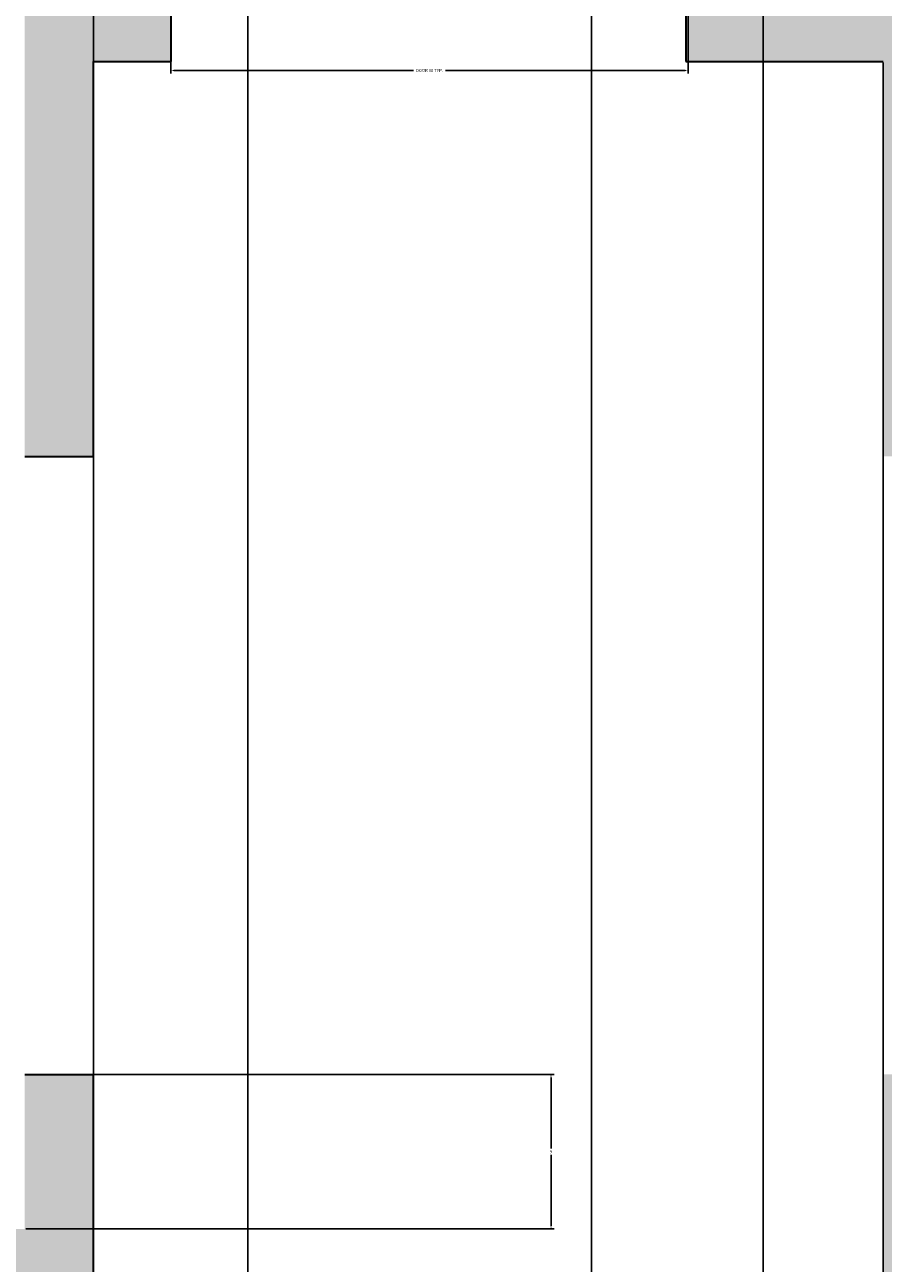
# Model space of a CAD drawing. Units: inches. Extents: x 1567 to 1964, y 1813 to 2447.
# Tile 24 of 28: x 1738 to 1788, y 2261 to 2333. Entities that reach past the tile are written whole.
import ezdxf

# ---------------------------------------------------------------- set-up
doc = ezdxf.new("R2010")
doc.units = ezdxf.units.IN
doc.layers.add('A-ANNO-DIMS', color=2, linetype='Continuous', lineweight=18)
doc.layers.add('A-WALL', color=7, linetype='Continuous', lineweight=35)
doc.layers.add('A-WALL-PATT', color=251, linetype='Continuous', lineweight=13, true_color=0x636466)
doc.styles.get("Standard").update_dxf_attribs({"font": 'arial.ttf'})
doc.dimstyles.get("Standard").update_dxf_attribs({"dimtxt": 0.18, "dimasz": 0.18, "dimexe": 0.18, "dimexo": 0.0625, "dimgap": 0.09, "dimtad": 0, "dimtih": 1, "dimtoh": 1, "dimdec": 4, "dimzin": 0, "dimdsep": 46, "dimtxsty": 'Standard', "dimcen": 0.09, "dimadec": 0, "dimazin": 0, "dimtfac": 1, "dimtdec": 4, "dimtofl": 0, "dimtmove": 0, "dimatfit": 3, "dimfxl": 1, "dimtolj": 1, "dimtzin": 0, "dimarcsym": 0})

# ---------------------------------------------------------------- blocks, each defined once
blk = doc.blocks.new('*D31')
at = {"layer": 'A-ANNO-DIMS', "color": 0, "lineweight": -2, "transparency": 16777216}
for p, q in [((1746.93, 2335.227), (1746.93, 2330.59)), ((1777.065, 2335.227), (1777.065, 2330.59)), ((1747.11, 2330.77), (1761.062, 2330.77)), ((1776.885, 2330.77), (1762.933, 2330.77))]:
    blk.add_line(p, q, dxfattribs=at)
at = {"layer": 'A-ANNO-DIMS', "color": 0, "transparency": 16777216}
for points in [[(1747.11, 2330.8), (1747.11, 2330.74), (1746.93, 2330.77)], [(1776.885, 2330.8), (1776.885, 2330.74), (1777.065, 2330.77)]]:
    blk.add_solid(points, dxfattribs=at)
at = {"layer": 'Defpoints', "color": 0, "transparency": 16777216}
for p in [(1746.93, 2335.29), (1777.065, 2335.29), (1777.065, 2330.77)]:
    blk.add_point(p, dxfattribs=at)
at = {"layer": 'A-ANNO-DIMS', "color": 0, "transparency": 16777216, "insert": (1761.997, 2330.77), "char_height": 0.18, "attachment_point": 5}
blk.add_mtext('\\A1;DOOR 30 TYP.', dxfattribs=at)
blk = doc.blocks.new('*D47')
at = {"layer": 'A-ANNO-DIMS', "color": 0, "lineweight": -2, "transparency": 16777216}
for p, q in [((1742.43, 2331.227), (1742.43, 1813.46)), ((1788.43, 2331.227), (1788.43, 1813.46)), ((1742.61, 1813.64), (1765.207, 1813.64)), ((1788.25, 1813.64), (1765.652, 1813.64))]:
    blk.add_line(p, q, dxfattribs=at)
at = {"layer": 'A-ANNO-DIMS', "color": 0, "transparency": 16777216}
for points in [[(1742.61, 1813.67), (1742.61, 1813.61), (1742.43, 1813.64)], [(1788.25, 1813.67), (1788.25, 1813.61), (1788.43, 1813.64)]]:
    blk.add_solid(points, dxfattribs=at)
at = {"layer": 'Defpoints', "color": 0, "transparency": 16777216}
for p in [(1742.43, 2331.29), (1788.43, 2331.29), (1788.43, 1813.64)]:
    blk.add_point(p, dxfattribs=at)
at = {"layer": 'A-ANNO-DIMS', "color": 0, "transparency": 16777216, "insert": (1765.43, 1813.64), "char_height": 0.18, "attachment_point": 5}
blk.add_mtext('\\A1;46', dxfattribs=at)
blk = doc.blocks.new('*D54')
at = {"layer": 'A-ANNO-DIMS', "color": 0, "lineweight": -2, "transparency": 16777216}
for p, q in [((1711.43, 1964.352), (1711.43, 2447.12)), ((1795.43, 1964.352), (1795.43, 2447.12)), ((1711.61, 2446.94), (1753.211, 2446.94)), ((1795.25, 2446.94), (1753.648, 2446.94))]:
    blk.add_line(p, q, dxfattribs=at)
at = {"layer": 'A-ANNO-DIMS', "color": 0, "transparency": 16777216}
for points in [[(1711.61, 2446.97), (1711.61, 2446.91), (1711.43, 2446.94)], [(1795.25, 2446.97), (1795.25, 2446.91), (1795.43, 2446.94)]]:
    blk.add_solid(points, dxfattribs=at)
at = {"layer": 'Defpoints', "color": 0, "transparency": 16777216}
for p in [(1795.43, 2446.94), (1711.43, 1964.29), (1795.43, 1964.29)]:
    blk.add_point(p, dxfattribs=at)
at = {"layer": 'A-ANNO-DIMS', "color": 0, "transparency": 16777216, "insert": (1753.43, 2446.94), "char_height": 0.18, "attachment_point": 5}
blk.add_mtext('\\A1;84', dxfattribs=at)
blk = doc.blocks.new('*D58')
at = {"layer": 'A-ANNO-DIMS', "color": 0, "lineweight": -2, "transparency": 16777216}
for p, q in [((1742.43, 2127.352), (1742.43, 2447.12)), ((1751.43, 2127.352), (1751.43, 2447.12)), ((1742.61, 2446.94), (1746.78, 2446.94)), ((1751.25, 2446.94), (1747.079, 2446.94))]:
    blk.add_line(p, q, dxfattribs=at)
at = {"layer": 'A-ANNO-DIMS', "color": 0, "transparency": 16777216}
for points in [[(1742.61, 2446.97), (1742.61, 2446.91), (1742.43, 2446.94)], [(1751.25, 2446.97), (1751.25, 2446.91), (1751.43, 2446.94)]]:
    blk.add_solid(points, dxfattribs=at)
at = {"layer": 'Defpoints', "color": 0, "transparency": 16777216}
for p in [(1751.43, 2446.94), (1742.43, 2127.29), (1751.43, 2127.29)]:
    blk.add_point(p, dxfattribs=at)
at = {"layer": 'A-ANNO-DIMS', "color": 0, "transparency": 16777216, "insert": (1746.93, 2446.94), "char_height": 0.18, "attachment_point": 5}
blk.add_mtext('\\A1;9', dxfattribs=at)
blk = doc.blocks.new('*D59')
at = {"layer": 'A-ANNO-DIMS', "color": 0, "lineweight": -2, "transparency": 16777216}
for p, q in [((1751.43, 2127.352), (1751.43, 2447.12)), ((1781.43, 2127.352), (1781.43, 2447.12)), ((1751.61, 2446.94), (1766.211, 2446.94)), ((1781.25, 2446.94), (1766.648, 2446.94))]:
    blk.add_line(p, q, dxfattribs=at)
at = {"layer": 'A-ANNO-DIMS', "color": 0, "transparency": 16777216}
for points in [[(1751.61, 2446.97), (1751.61, 2446.91), (1751.43, 2446.94)], [(1781.25, 2446.97), (1781.25, 2446.91), (1781.43, 2446.94)]]:
    blk.add_solid(points, dxfattribs=at)
at = {"layer": 'Defpoints', "color": 0, "transparency": 16777216}
for p in [(1781.43, 2446.94), (1751.43, 2127.29), (1781.43, 2127.29)]:
    blk.add_point(p, dxfattribs=at)
at = {"layer": 'A-ANNO-DIMS', "color": 0, "transparency": 16777216, "insert": (1766.43, 2446.94), "char_height": 0.18, "attachment_point": 5}
blk.add_mtext('\\A1;30', dxfattribs=at)
blk = doc.blocks.new('*D63')
at = {"layer": 'A-ANNO-DIMS', "color": 0, "lineweight": -2, "transparency": 16777216}
for p, q in [((1735.43, 1988.352), (1735.43, 2447.12)), ((1771.43, 1988.352), (1771.43, 2447.12)), ((1735.61, 2446.94), (1753.211, 2446.94)), ((1771.25, 2446.94), (1753.648, 2446.94))]:
    blk.add_line(p, q, dxfattribs=at)
at = {"layer": 'A-ANNO-DIMS', "color": 0, "transparency": 16777216}
for points in [[(1735.61, 2446.97), (1735.61, 2446.91), (1735.43, 2446.94)], [(1771.25, 2446.97), (1771.25, 2446.91), (1771.43, 2446.94)]]:
    blk.add_solid(points, dxfattribs=at)
at = {"layer": 'Defpoints', "color": 0, "transparency": 16777216}
for p in [(1771.43, 2446.94), (1735.43, 1988.29), (1771.43, 1988.29)]:
    blk.add_point(p, dxfattribs=at)
at = {"layer": 'A-ANNO-DIMS', "color": 0, "transparency": 16777216, "insert": (1753.43, 2446.94), "char_height": 0.18, "attachment_point": 5}
blk.add_mtext('\\A1;36', dxfattribs=at)
blk = doc.blocks.new('*D68')
at = {"layer": 'A-ANNO-DIMS', "color": 0, "lineweight": -2, "transparency": 16777216}
for p, q in [((1738.492, 2272.29), (1769.26, 2272.29)), ((1769.08, 2272.11), (1769.08, 2267.972)), ((1769.08, 2263.47), (1769.08, 2267.608)), ((1738.492, 2263.29), (1769.26, 2263.29))]:
    blk.add_line(p, q, dxfattribs=at)
at = {"layer": 'A-ANNO-DIMS', "color": 0, "transparency": 16777216}
for points in [[(1769.05, 2272.11), (1769.11, 2272.11), (1769.08, 2272.29)], [(1769.05, 2263.47), (1769.11, 2263.47), (1769.08, 2263.29)]]:
    blk.add_solid(points, dxfattribs=at)
at = {"layer": 'Defpoints', "color": 0, "transparency": 16777216}
for p in [(1738.43, 2272.29), (1738.43, 2263.29), (1769.08, 2263.29)]:
    blk.add_point(p, dxfattribs=at)
at = {"layer": 'A-ANNO-DIMS', "color": 0, "transparency": 16777216, "insert": (1769.08, 2267.79), "char_height": 0.18, "attachment_point": 5}
blk.add_mtext('\\A1;9', dxfattribs=at)

msp = doc.modelspace()

# ---------------------------------------------------------------- hatches: boundary and pattern name
at = {"layer": 'A-WALL-PATT'}
h = msp.add_hatch(color=256, dxfattribs=at)
h.dxf.hatch_style = 1
h.paths.add_polyline_path([(1606.4295, 2407.29), (1654.4295, 2407.29), (1654.4295, 2416.29), (1597.4295, 2416.29), (1597.4295, 2217.29), (1606.4295, 2217.29), (1606.4295, 2259.29), (1738.4295, 2259.29), (1738.4295, 2247.29), (1742.4295, 2247.29), (1742.4295, 2259.29), (1742.4295, 2272.29), (1738.4295, 2272.29), (1738.4295, 2263.29), (1606.4295, 2263.29)])
h.paths.add_polyline_path([(1753.4295, 2416.29), (1690.4295, 2416.29), (1690.4295, 2407.29), (1738.4295, 2407.29), (1738.4295, 2308.29), (1742.4295, 2308.29), (1742.4295, 2331.29), (1746.9295, 2331.29), (1746.9295, 2335.29), (1742.4295, 2335.29), (1742.4295, 2407.29), (1753.4295, 2407.29)])
h.paths.add_polyline_path([(1840.4295, 2416.29), (1777.4295, 2416.29), (1777.4295, 2407.29), (1788.4295, 2407.29), (1788.4295, 2335.29), (1776.9295, 2335.29), (1776.9295, 2331.29), (1788.4295, 2331.29), (1788.4295, 2308.29), (1792.4295, 2308.29), (1792.4295, 2407.29), (1840.4295, 2407.29)])
h.paths.add_polyline_path([(1933.4295, 2416.29), (1876.4295, 2416.29), (1876.4295, 2407.29), (1924.4295, 2407.29), (1924.4295, 2263.29), (1792.4295, 2263.29), (1792.4295, 2272.29), (1788.4295, 2272.29), (1788.4295, 2259.29), (1872.4295, 2259.29), (1872.4295, 2171.29), (1880.9295, 2171.29), (1880.9295, 2175.29), (1876.4295, 2175.29), (1876.4295, 2259.29), (1924.4295, 2259.29), (1924.4295, 2229.29), (1933.4295, 2229.29)])
h.paths.add_polyline_path([(1933.4295, 2205.29), (1924.4295, 2205.29), (1924.4295, 2175.29), (1910.9295, 2175.29), (1910.9295, 2171.29), (1924.4295, 2171.29), (1924.4295, 2127.29), (1844.4295, 2127.29), (1844.4295, 2123.29), (1924.4295, 2123.29), (1924.4295, 2063.29), (1933.4295, 2063.29)])
h.paths.add_polyline_path([(1799.4295, 2123.29), (1808.4295, 2123.29), (1808.4295, 2127.29), (1781.4295, 2127.29), (1781.4295, 2123.29), (1795.4295, 2123.29), (1795.4295, 1964.29), (1711.4295, 1964.29), (1711.4295, 2123.29), (1751.4295, 2123.29), (1751.4295, 2127.29), (1742.4295, 2127.29), (1742.4295, 2139.29), (1738.4295, 2139.29), (1738.4295, 2127.29), (1678.4295, 2127.29), (1678.4295, 2123.29), (1702.4295, 2123.29), (1702.4295, 1913.29), (1678.4295, 1913.29), (1678.4295, 1904.29), (1711.4295, 1904.29), (1711.4295, 1960.29), (1795.4295, 1960.29), (1795.4295, 1906.69), (1929.4295, 1906.69), (1929.4295, 1848.29), (1601.4295, 1848.29), (1601.4295, 1904.29), (1630.4295, 1904.29), (1630.4295, 1913.29), (1606.4295, 1913.29), (1606.4295, 2123.29), (1630.4295, 2123.29), (1630.4295, 2127.29), (1606.4295, 2127.29), (1606.4295, 2169.29), (1597.4295, 2169.29), (1597.4295, 1844.29), (1933.4295, 1844.29), (1933.4295, 2027.29), (1924.4295, 2027.29), (1924.4295, 1967.29), (1833.9295, 1967.29), (1833.9295, 1963.29), (1924.4295, 1963.29), (1924.4295, 1910.69), (1799.4295, 1910.69), (1799.4295, 1963.29), (1803.9295, 1963.29), (1803.9295, 1967.29), (1799.4295, 1967.29)])

# ---------------------------------------------------------------- linework, layer by layer
at = {"layer": 'A-WALL'}
for p, q in [((1746.9295, 2335.29), (1746.9295, 2331.29)), ((1776.9295, 2335.29), (1776.9295, 2331.29)), ((1742.4295, 2331.29), (1746.9295, 2331.29)), ((1742.4295, 2308.29), (1742.4295, 2331.29)), ((1776.9295, 2331.29), (1788.4295, 2331.29)), ((1738.4295, 2308.29), (1742.4295, 2308.29)), ((1738.4295, 2272.29), (1742.4295, 2272.29)), ((1742.4295, 2259.29), (1742.4295, 2272.29))]:
    msp.add_line(p, q, dxfattribs=at)

# ---------------------------------------------------------------- dimensions: what is measured, and where the dimension line sits
at = {"layer": 'A-ANNO-DIMS'}
for base, p1, p2, picture, middle in [((1795.4295, 2446.94), (1711.4295, 1964.29), (1795.4295, 1964.29), '*D54', (1753.4295, 2446.94)), ((1771.4295, 2446.94), (1735.4295, 1988.29), (1771.4295, 1988.29), '*D63', (1753.4295, 2446.94)), ((1751.4295, 2446.94), (1742.4295, 2127.29), (1751.4295, 2127.29), '*D58', (1746.9295, 2446.94)), ((1781.4295, 2446.94), (1751.4295, 2127.29), (1781.4295, 2127.29), '*D59', (1766.4295, 2446.94)), ((1788.4295, 1813.64), (1742.4295, 2331.29), (1788.4295, 2331.29), '*D47', (1765.4295, 1813.64))]:
    dim = msp.add_linear_dim(base=base, p1=p1, p2=p2, dimstyle='Standard', override={"dimdec": 0, "dimlfac": 1, "dimrnd": 0, "dimzin": 0, "dimdsep": 46, "dimlunit": 2}, dxfattribs=at)
    dim.commit()
    dim.dimension.update_dxf_attribs({"geometry": picture, "text_midpoint": middle})
dim = msp.add_linear_dim(base=(1777.0651, 2330.7697), p1=(1746.9295, 2335.29), p2=(1777.0651, 2335.29), text='DOOR <> TYP.', dimstyle='Standard', override={"dimdec": 0, "dimlfac": 1, "dimrnd": 0, "dimzin": 0, "dimdsep": 46, "dimlunit": 2}, dxfattribs=at)
dim.commit()
dim.dimension.update_dxf_attribs({"geometry": '*D31', "text_midpoint": (1761.9973, 2330.7697)})
dim = msp.add_linear_dim(base=(1769.0795, 2263.29), p1=(1738.4295, 2272.29), p2=(1738.4295, 2263.29), angle=270, dimstyle='Standard', override={"dimdec": 0, "dimlfac": 1, "dimrnd": 0, "dimzin": 0, "dimdsep": 46, "dimlunit": 2}, dxfattribs=at)
dim.commit()
dim.dimension.update_dxf_attribs({"geometry": '*D68', "text_midpoint": (1769.0795, 2267.79)})

doc.saveas('drawing.dxf')
